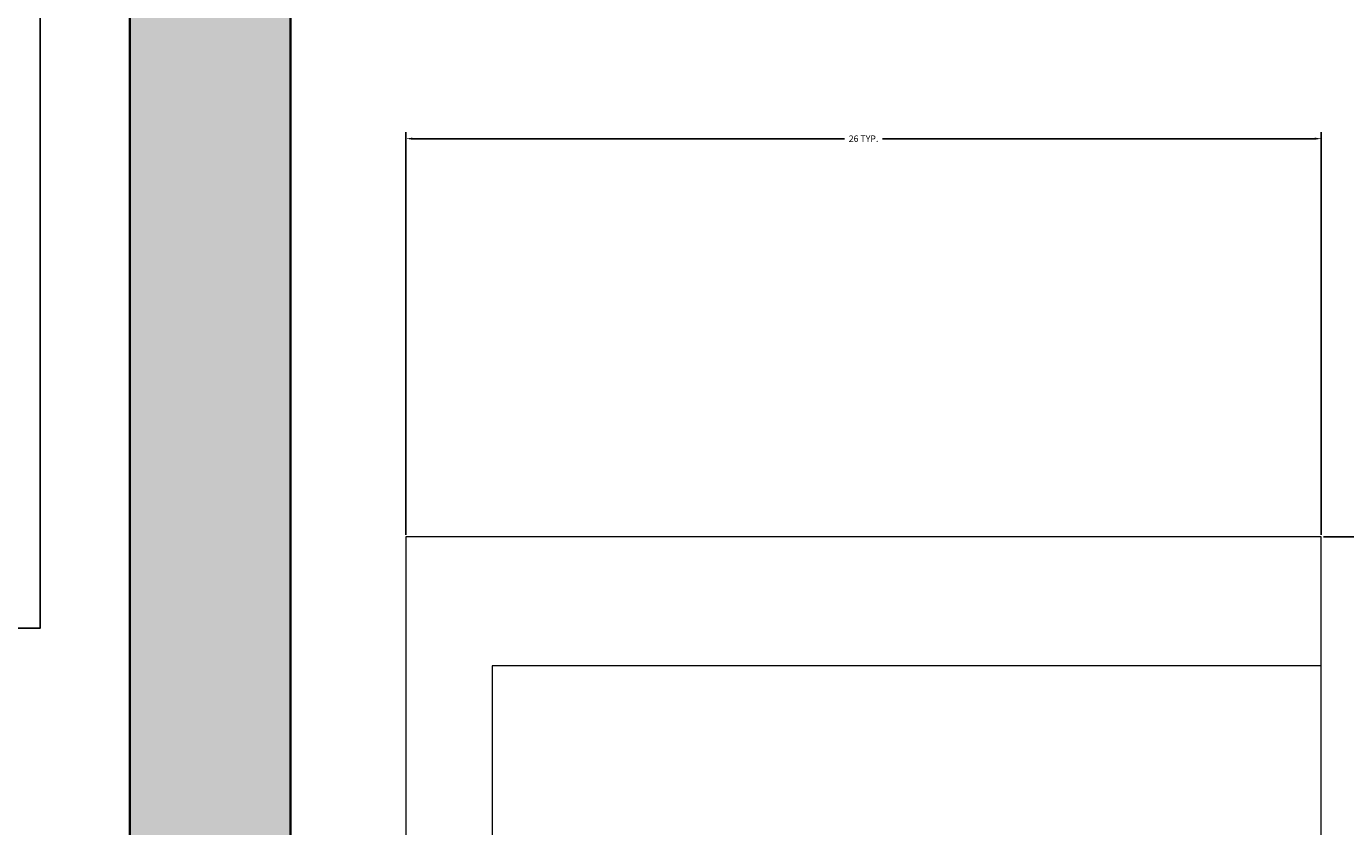
# Model space of a CAD drawing. Units: inches. Extents: x 1998 to 2588, y 1139 to 1977.
# Tile 53 of 134: x 2220 to 2257, y 1663 to 1686. Entities that reach past the tile are written whole.
import ezdxf

# ---------------------------------------------------------------- set-up
doc = ezdxf.new("R2010")
doc.units = ezdxf.units.IN
for name, color, linetype, lineweight in [('A-ANNO-DIMS', 2, 'Continuous', 18), ('A-WALL-PATT', 252, 'Continuous', 13), ('DOOR', 52, 'Continuous', 25), ('FUR', 21, 'Continuous', 18), ('WALL', 200, 'Continuous', 35)]:
    doc.layers.add(name, color=color, linetype=linetype, lineweight=lineweight)
doc.styles.get("Standard").update_dxf_attribs({"font": 'arial.ttf'})
doc.dimstyles.get("Standard").update_dxf_attribs({"dimtxt": 0.18, "dimasz": 0.18, "dimexe": 0.18, "dimexo": 0.0625, "dimgap": 0.09, "dimtad": 0, "dimtih": 1, "dimtoh": 1, "dimdec": 4, "dimzin": 0, "dimdsep": 46, "dimtxsty": 'Standard', "dimcen": 0.09, "dimadec": 0, "dimazin": 0, "dimtfac": 1, "dimtdec": 4, "dimtofl": 0, "dimtmove": 0, "dimatfit": 3, "dimfxl": 1, "dimtolj": 1, "dimtzin": 0, "dimarcsym": 0})

# ---------------------------------------------------------------- blocks, each defined once
blk = doc.blocks.new('*U2')
for p, q in [((0, 0), (0, -6)), ((40, 0), (40, -6))]:
    blk.add_line(p, q)
blk.add_lwpolyline([(0, 0), (0, 40), (1.75, 40), (1.75, 0)], close=True)
blk.add_arc((0, 0), 40, 0, 90)
blk = doc.blocks.new('SOFA-THREE-SEAT')
for p, q in [((3.604, 25.615), (0, 25.615)), ((0, 25.615), (0, 0)), ((0, 0), (74.336, 0))]:
    blk.add_line(p, q)
blk.add_lwpolyline([(3.604, 2.416), (71.008, 2.416), (71.008, 25.615), (3.604, 25.615)], close=True)
blk = doc.blocks.new('*D11')
at = {"layer": 'A-ANNO-DIMS', "color": 0, "lineweight": -2, "transparency": 16777216}
for p, q in [((2256.378, 1671.356), (2267.646, 1671.356)), ((2267.466, 1671.176), (2267.466, 1634.372)), ((2267.466, 1597.201), (2267.466, 1634.005)), ((2256.378, 1597.021), (2267.646, 1597.021))]:
    blk.add_line(p, q, dxfattribs=at)
at = {"layer": 'A-ANNO-DIMS', "color": 0, "transparency": 16777216}
for points in [[(2267.436, 1671.176), (2267.496, 1671.176), (2267.466, 1671.356)], [(2267.436, 1597.201), (2267.496, 1597.201), (2267.466, 1597.021)]]:
    blk.add_solid(points, dxfattribs=at)
at = {"layer": 'Defpoints', "color": 0, "transparency": 16777216}
for p in [(2256.316, 1671.356), (2256.316, 1597.021), (2267.466, 1597.021)]:
    blk.add_point(p, dxfattribs=at)
at = {"layer": 'A-ANNO-DIMS', "color": 0, "transparency": 16777216, "insert": (2267.466, 1634.189), "char_height": 0.18, "attachment_point": 5}
blk.add_mtext('\\A1;SOFA 74 TYP.', dxfattribs=at)
blk = doc.blocks.new('*D12')
at = {"layer": 'A-ANNO-DIMS', "color": 0, "lineweight": -2, "transparency": 16777216}
for p, q in [((2230.701, 1671.419), (2230.701, 1682.687)), ((2230.881, 1682.507), (2242.979, 1682.507)), ((2256.136, 1682.507), (2244.038, 1682.507)), ((2256.316, 1671.419), (2256.316, 1682.687))]:
    blk.add_line(p, q, dxfattribs=at)
at = {"layer": 'A-ANNO-DIMS', "color": 0, "transparency": 16777216}
for points in [[(2230.881, 1682.537), (2230.881, 1682.477), (2230.701, 1682.507)], [(2256.136, 1682.537), (2256.136, 1682.477), (2256.316, 1682.507)]]:
    blk.add_solid(points, dxfattribs=at)
at = {"layer": 'Defpoints', "color": 0, "transparency": 16777216}
for p in [(2256.316, 1682.507), (2230.701, 1671.356), (2256.316, 1671.356)]:
    blk.add_point(p, dxfattribs=at)
at = {"layer": 'A-ANNO-DIMS', "color": 0, "transparency": 16777216, "insert": (2243.508, 1682.507), "char_height": 0.18, "attachment_point": 5}
blk.add_mtext('\\A1;26 TYP.', dxfattribs=at)
blk = doc.blocks.new('*D36')
at = {"layer": 'A-ANNO-DIMS', "color": 0, "lineweight": -2, "transparency": 16777216}
for p, q in [((2197.45, 1663.309), (2197.45, 1977.362)), ((2197.63, 1977.182), (2209.746, 1977.182)), ((2222.793, 1977.182), (2210.677, 1977.182)), ((2222.973, 1663.309), (2222.973, 1977.362))]:
    blk.add_line(p, q, dxfattribs=at)
at = {"layer": 'A-ANNO-DIMS', "color": 0, "transparency": 16777216}
for points in [[(2197.63, 1977.212), (2197.63, 1977.152), (2197.45, 1977.182)], [(2222.793, 1977.212), (2222.793, 1977.152), (2222.973, 1977.182)]]:
    blk.add_solid(points, dxfattribs=at)
at = {"layer": 'Defpoints', "color": 0, "transparency": 16777216}
for p in [(2222.973, 1977.182), (2197.45, 1663.247), (2222.973, 1663.247)]:
    blk.add_point(p, dxfattribs=at)
at = {"layer": 'A-ANNO-DIMS', "color": 0, "transparency": 16777216, "insert": (2210.211, 1977.182), "char_height": 0.18, "attachment_point": 5}
blk.add_mtext('\\A1;25.523', dxfattribs=at)

msp = doc.modelspace()

# ---------------------------------------------------------------- hatches: boundary and pattern name
at = {"layer": 'A-WALL-PATT'}
h = msp.add_hatch(color=256, dxfattribs=at)
h.dxf.hatch_style = 1
h.paths.add_polyline_path([(2527.4729, 1362.2324), (2510.9729, 1362.2324), (2510.9729, 1357.7324), (2518.4729, 1357.7324), (2518.4729, 1237.7324), (2503.1458, 1237.7324), (2503.1458, 1228.7324), (2527.4729, 1228.7324)])
h.paths.add_polyline_path([(2490.5682, 1362.2324), (2398.4729, 1362.2324), (2398.4729, 1357.7324), (2490.5682, 1357.7324)])
h.paths.add_polyline_path([(2224.9729, 1264.7324), (2222.9729, 1264.7324), (2222.9729, 1232.4125), (2341.4729, 1232.4125), (2341.4729, 1234.4125), (2224.9729, 1234.4125)])
h.paths.add_polyline_path([(2334.5332, 1273.7324), (2264.7638, 1273.7324), (2264.7638, 1269.5611, -0.043659), (2264.3413, 1264.7324), (2334.5332, 1264.7324)])
h.paths.add_polyline_path([(2236.9551, 1273.7324), (2234.4125, 1273.7324), (2234.4125, 1264.7324), (2236.9551, 1264.7324), (2236.9551, 1269.5611)])
h.paths.add_polyline_path([(2222.9729, 1293.2324), (2096.9729, 1293.2324), (2096.9729, 1345.0966), (2087.9729, 1345.0966), (2087.9729, 1284.2324), (2222.9729, 1284.2324), (2222.9729, 1285.137)])
h.paths.add_polyline_path([(2096.9729, 1458.7927), (2087.9729, 1458.7927), (2087.9729, 1417.7324), (2087.9729, 1413.2324), (2096.9729, 1413.2324), (2096.9729, 1417.7324)])
h.paths.add_polyline_path([(2096.9729, 1413.2324), (2087.9729, 1413.2324), (2087.9729, 1365.5012), (2096.9729, 1365.5012), (2096.9729, 1369.3358)])
h.paths.add_polyline_path([(2186.2943, 1417.7324), (2138.6074, 1417.7324), (2096.9729, 1417.7324), (2096.9729, 1413.2324), (2138.6074, 1413.2324), (2186.2943, 1413.2324)])
h.paths.add_polyline_path([(2181.4729, 1465.7324), (2176.9729, 1465.7324), (2176.9729, 1451.6434), (2181.4729, 1451.6434)])
h.paths.add_polyline_path([(2181.4729, 1422.1664), (2176.9729, 1422.1664), (2176.9729, 1417.7324), (2181.4729, 1417.7324)])
h.paths.add_polyline_path([(2063.9729, 1465.7324), (2087.9729, 1465.7324), (2087.9729, 1470.2324), (2059.4729, 1470.2324), (2059.4729, 1413.2324), (2087.9729, 1413.2324), (2087.9729, 1417.7324), (2063.9729, 1417.7324)])
h.paths.add_polyline_path([(2181.4729, 1755.2324), (2176.9729, 1755.2324), (2176.9729, 1748.6798), (2177.0513, 1748.6798), (2181.4729, 1748.6798)])
h.paths.add_polyline_path([(2227.4729, 1707.2324), (2220.4647, 1707.2324), (2220.4647, 1702.7324), (2222.9729, 1702.7324), (2222.9729, 1604.637), (2227.4729, 1604.637)])
h.paths.add_polyline_path([(2114.9729, 1702.7324), (2105.9729, 1702.7324), (2105.9729, 1628.4781, -0.0318759), (2110.1012, 1628.7416), (2114.9729, 1628.7416)])
h.paths.add_polyline_path([(2345.9729, 1739.3278), (2341.4729, 1739.3278), (2341.4729, 1647.5211), (2345.9729, 1647.5211)])
h.paths.add_polyline_path([(2350.6273, 1641.2324), (2345.9729, 1641.2324), (2345.9729, 1636.7324), (2350.6273, 1636.7324), (2350.6273, 1639.8729)])
h.paths.add_polyline_path([(2501.9729, 1641.2324), (2407.9729, 1641.2324), (2392.5005, 1641.2324), (2392.5005, 1639.8729), (2392.5005, 1636.7324), (2501.9729, 1636.7324)])
h.paths.add_polyline_path([(2510.9729, 1755.2324), (2501.9729, 1755.2324), (2501.9729, 1641.2324), (2510.9729, 1641.2324)])
h.paths.add_polyline_path([(2549.1786, 1641.2324), (2522.3775, 1641.2324), (2522.3775, 1636.7324), (2540.1786, 1636.7324), (2540.1786, 1480.7324), (2522.3775, 1480.7324), (2522.3775, 1476.2324), (2549.1786, 1476.2324)])
h.paths.add_polyline_path([(2498.1786, 1594.7324), (2407.9729, 1594.7324), (2407.9729, 1585.7324), (2416.9729, 1585.7324), (2489.1786, 1585.7324), (2489.1786, 1531.7324), (2416.9729, 1531.7324), (2407.9729, 1531.7324), (2407.9729, 1522.7324), (2498.1786, 1522.7324)])
h.paths.add_polyline_path([(2351.6437, 1480.7324), (2345.9729, 1480.7324), (2345.9729, 1476.2324), (2351.6437, 1476.2324), (2351.6437, 1477.5919)])
h.paths.add_polyline_path([(2501.9729, 1480.7324), (2498.1786, 1480.7324), (2407.9729, 1480.7324), (2393.5168, 1480.7324), (2393.5168, 1477.5919), (2393.5168, 1476.2324), (2501.9729, 1476.2324)])

# ---------------------------------------------------------------- linework, layer by layer
at = {"layer": 'WALL'}
for p, q in [((2227.4729, 1707.2324), (2227.4729, 1584.2324)), ((2222.9729, 1702.7324), (2222.9729, 1604.637))]:
    msp.add_line(p, q, dxfattribs=at)

# ---------------------------------------------------------------- block references
at = {"layer": 'DOOR', "xscale": 0.8354643497673233, "yscale": 0.8354643497673233, "zscale": 0.8354643497673233, "rotation": 180}
msp.add_blockref('*U2', (2220.4647, 1702.2196), dxfattribs=at)
at = {"layer": 'FUR', "rotation": 270.0000000000001}
msp.add_blockref('SOFA-THREE-SEAT', (2230.701, 1671.3567), dxfattribs=at)

# ---------------------------------------------------------------- dimensions: what is measured, and where the dimension line sits
at = {"layer": 'A-ANNO-DIMS'}
dim = msp.add_linear_dim(base=(2222.9729, 1977.1824), p1=(2197.4499, 1663.2466), p2=(2222.9729, 1663.2466), dimstyle='Standard', override={"dimdec": 3, "dimlfac": 1, "dimrnd": 0, "dimzin": 0, "dimdsep": 46, "dimlunit": 2}, dxfattribs=at)
dim.commit()
dim.dimension.update_dxf_attribs({"geometry": '*D36', "text_midpoint": (2210.2114, 1977.1824)})
dim = msp.add_linear_dim(base=(2256.3158, 1682.5069), p1=(2230.7007, 1671.3565), p2=(2256.3158, 1671.3565), text='<> TYP.', dimstyle='Standard', override={"dimdec": 0, "dimlfac": 1, "dimrnd": 0, "dimzin": 0, "dimdsep": 46, "dimlunit": 2}, dxfattribs=at)
dim.commit()
dim.dimension.update_dxf_attribs({"geometry": '*D12', "text_midpoint": (2243.5082, 1682.5069)})
dim = msp.add_linear_dim(base=(2267.4662, 1597.0205), p1=(2256.3158, 1671.3565), p2=(2256.3158, 1597.0205), angle=270, text='SOFA <> TYP.', dimstyle='Standard', override={"dimdec": 0, "dimlfac": 1, "dimrnd": 0, "dimzin": 0, "dimdsep": 46, "dimlunit": 2}, dxfattribs=at)
dim.commit()
dim.dimension.update_dxf_attribs({"geometry": '*D11', "text_midpoint": (2267.4662, 1634.1885)})

doc.saveas('drawing.dxf')
